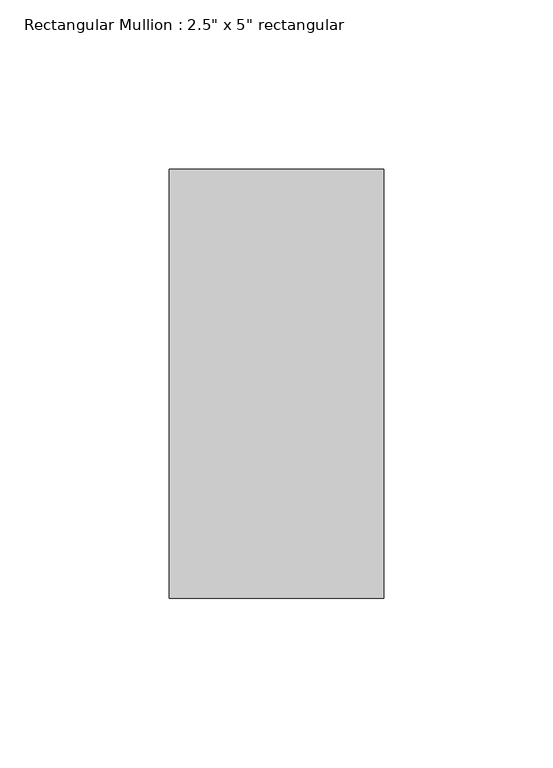
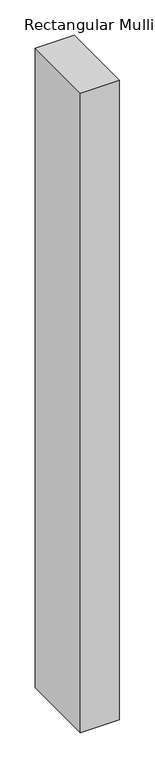
"""IFC4 building model written with IfcOpenShell, lengths in millimetres: member geometry."""

from ifc_helpers import new_model, si_unit, frame, origin, place, context, project, spatial, polyline, outline, extrude, source, transform, mapped, element, save


def member_240932ed(model_context):
    return source(origin(), model_context, "Body", "SweptSolid", [
        extrude(outline(polyline([(0.0, 63.5), (0.0, -63.5), (-63.5, -63.5), (-63.5, 63.5), (0.0, 63.5)])), frame((0.0, 0.0, -1100.6666665), z_axis=(0.0, 0.0, 1.0), x_axis=(1.0, 0.0, 0.0)), (0.0, 0.0, 1.0), 1100.6666665),
    ])


if __name__ == "__main__":
    model = new_model("IFC4")
    model_context = context("Model", 3, world=origin())
    ifc_project = project(units=[si_unit("LENGTHUNIT", "METRE", prefix="MILLI")], contexts=[model_context])
    site = spatial("IfcSite", under=ifc_project)
    building = spatial("IfcBuilding", under=site)
    placement = place(None, origin())
    member_shape = member_240932ed(model_context)
    element("IfcMember", 1, ObjectType="Rectangular Mullion : 2.5\" x 5\" rectangular", at=placement, inside=building, context=model_context, shape_type="MappedRepresentation", body=[
        mapped(member_shape, transform((0.0, 0.0, 0.0), x_axis=(1.0, 0.0, 0.0), y_axis=(0.0, 1.0, 0.0), z_axis=(0.0, 0.0, 1.0))),
    ])
    save(model, "model.ifc")

# Revit data of these elements
# Type "Rectangular Mullion : 2.5\" x 5\" rectangular"
#   built-in parameter 1007304 = 0.416667 (stored number, unit not read)
#   built-in parameter 1007301 = 0.104167 (stored number, unit not read)
#   built-in parameter 1007300 = 0.104167 (stored number, unit not read)
# Element 1 (IfcMember, "Rectangular Mullion : 2.5\" x 5\" rectangular")
#   Materials on its faces: "metal black"
# Materials
#   "metal black": class "Generic", colour RGB 120 120 120, transparency 0, Cost = 0
